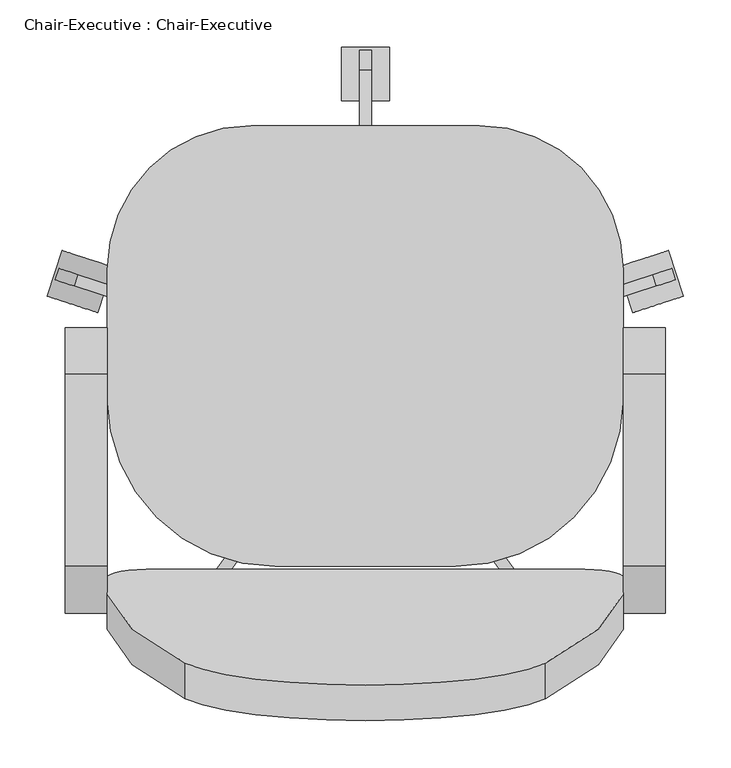
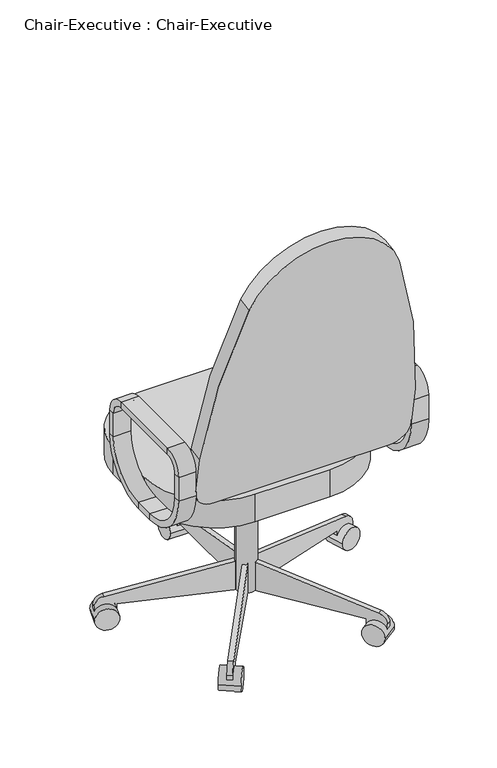
"""IFC4 building model written with IfcOpenShell, lengths in millimetres: furniture geometry, Chair-Executive : Chair-Executive."""

from ifc_helpers import new_model, si_unit, point, frame, frame_2d, origin, place, context, project, spatial, polyline, circle_curve, trimmed, segment, composite_curve, outline, extrude, source, transform, mapped, element, save
from ifc_brep_helpers import plane_surface, cylinder_surface, revolved_surface, advanced_brep


def chair_executive_chair_executive_8d69e98c(model_context):
    return source(origin(), model_context, "Body", "SolidModel", [
        advanced_brep(
        [(-176.5091803, -217.7873012, 546.1), (-176.5091803, -108.0540984, 436.3667972), (-176.5091803, -108.0540984, 420.4917972), (-176.5091803, -233.6623012, 546.1), (-132.0591803, -217.7873012, 546.1), (-132.0591803, -108.0540984, 436.3667972), (-132.0591803, -233.6623012, 546.1), (-132.0591803, -108.0540984, 420.4917972), (-176.5091803, -233.6623012, 609.6), (-176.5091803, -217.7873012, 609.6), (-132.0591803, -217.7873012, 609.6), (-132.0591803, -233.6623012, 609.6), (-176.5091803, -184.2540984, 643.1332028), (-176.5091803, -184.2540984, 659.0082028), (-132.0591803, -184.2540984, 643.1332028), (-132.0591803, -184.2540984, 659.0082028), (-176.5091803, 18.9459016, 659.0082028), (-176.5091803, 18.9459016, 643.1332028), (-132.0591803, 18.9459016, 643.1332028), (-132.0591803, 18.9459016, 659.0082028), (-176.5091803, 52.4791044, 609.6), (-176.5091803, 68.3541044, 609.6), (-132.0591803, 52.4791044, 609.6), (-132.0591803, 68.3541044, 609.6), (-176.5091803, 68.3541044, 546.1), (-176.5091803, 52.4791044, 546.1), (-132.0591803, 52.4791044, 546.1), (-132.0591803, 68.3541044, 546.1), (-176.5091803, -57.2540984, 436.3667972), (-176.5091803, -57.2540984, 420.4917972), (-132.0591803, -57.2540984, 436.3667972), (-132.0591803, -57.2540984, 420.4917972)],
        [
            (0, 1, circle_curve(frame((-176.5091803, -108.0540984, 546.1), z_axis=(1.0, 0.0, 0.0), x_axis=(0.0, 0.0, -1.0)), 109.7332028)),
            (1, 2),
            (2, 3, circle_curve(frame((-176.5091803, -108.0540984, 546.1), z_axis=(-1.0, 0.0, 0.0), x_axis=(0.0, 0.0, -1.0)), 125.6082028)),
            (3, 0),
            (4, 5, circle_curve(frame((-132.0591803, -108.0540984, 546.1), z_axis=(1.0, 0.0, 0.0), x_axis=(0.0, 0.0, -1.0)), 109.7332028)),
            (5, 1),
            (0, 4),
            (6, 7, circle_curve(frame((-132.0591803, -108.0540984, 546.1), z_axis=(1.0, 0.0, 0.0), x_axis=(0.0, 0.0, -1.0)), 125.6082028)),
            (7, 5),
            (4, 6),
            (2, 7),
            (6, 3),
            (3, 8),
            (8, 9),
            (9, 0),
            (9, 10),
            (10, 4),
            (10, 11),
            (11, 6),
            (11, 8),
            (12, 9, circle_curve(frame((-176.5091803, -184.2540984, 609.6), z_axis=(1.0, 0.0, 0.0), x_axis=(0.0, -1.0, 0.0)), 33.5332028)),
            (8, 13, circle_curve(frame((-176.5091803, -184.2540984, 609.6), z_axis=(-1.0, 0.0, 0.0), x_axis=(0.0, -1.0, 0.0)), 49.4082028)),
            (13, 12),
            (14, 10, circle_curve(frame((-132.0591803, -184.2540984, 609.6), z_axis=(1.0, 0.0, 0.0), x_axis=(0.0, -1.0, 0.0)), 33.5332028)),
            (12, 14),
            (15, 11, circle_curve(frame((-132.0591803, -184.2540984, 609.6), z_axis=(1.0, 0.0, 0.0), x_axis=(0.0, -1.0, 0.0)), 49.4082028)),
            (14, 15),
            (15, 13),
            (13, 16),
            (16, 17),
            (17, 12),
            (17, 18),
            (18, 14),
            (18, 19),
            (19, 15),
            (19, 16),
            (20, 17, circle_curve(frame((-176.5091803, 18.9459016, 609.6), z_axis=(1.0, 0.0, 0.0), x_axis=(0.0, 0.0, 1.0)), 33.5332028)),
            (16, 21, circle_curve(frame((-176.5091803, 18.9459016, 609.6), z_axis=(-1.0, 0.0, 0.0), x_axis=(0.0, 0.0, 1.0)), 49.4082028)),
            (21, 20),
            (22, 18, circle_curve(frame((-132.0591803, 18.9459016, 609.6), z_axis=(1.0, 0.0, 0.0), x_axis=(0.0, 0.0, 1.0)), 33.5332028)),
            (20, 22),
            (23, 19, circle_curve(frame((-132.0591803, 18.9459016, 609.6), z_axis=(1.0, 0.0, 0.0), x_axis=(0.0, 0.0, 1.0)), 49.4082028)),
            (22, 23),
            (23, 21),
            (21, 24),
            (24, 25),
            (25, 20),
            (25, 26),
            (26, 22),
            (26, 27),
            (27, 23),
            (27, 24),
            (28, 25, circle_curve(frame((-176.5091803, -57.2540984, 546.1), z_axis=(1.0, 0.0, 0.0), x_axis=(0.0, 1.0, 0.0)), 109.7332028)),
            (24, 29, circle_curve(frame((-176.5091803, -57.2540984, 546.1), z_axis=(-1.0, 0.0, 0.0), x_axis=(0.0, 1.0, 0.0)), 125.6082028)),
            (29, 28),
            (30, 26, circle_curve(frame((-132.0591803, -57.2540984, 546.1), z_axis=(1.0, 0.0, 0.0), x_axis=(0.0, 1.0, 0.0)), 109.7332028)),
            (28, 30),
            (31, 27, circle_curve(frame((-132.0591803, -57.2540984, 546.1), z_axis=(1.0, 0.0, 0.0), x_axis=(0.0, 1.0, 0.0)), 125.6082028)),
            (30, 31),
            (31, 29),
            (29, 2),
            (1, 28),
            (5, 30),
            (7, 31),
        ],
        [
            plane_surface(frame((-176.5091803, -108.0540984, 546.1), z_axis=(-1.0, 0.0, 0.0), x_axis=(0.0, 0.0, -1.0))),
            revolved_surface(polyline([(-176.5091803, -108.0540984, 436.3667972), (-132.0591803, -108.0540984, 436.3667972)]), (-132.0591803, -108.0540984, 546.1), (-1.0, 0.0, 0.0)),
            plane_surface(frame((-132.0591803, -108.0540984, 546.1), z_axis=(1.0, 0.0, 0.0), x_axis=(0.0, 0.0, -1.0))),
            cylinder_surface(frame((-132.0591803, -108.0540984, 546.1), z_axis=(-1.0, 0.0, 0.0), x_axis=(0.0, 0.0, -1.0)), 125.6082028),
            plane_surface(frame((-176.5091803, -233.6623012, 546.1), z_axis=(-1.0, 0.0, 0.0), x_axis=(0.0, 0.0, 1.0))),
            plane_surface(frame((-176.5091803, -217.7873012, 546.1), z_axis=(0.0, 1.0, 0.0), x_axis=(0.0, 0.0, 1.0))),
            plane_surface(frame((-132.0591803, -217.7873012, 546.1), z_axis=(1.0, 0.0, 0.0), x_axis=(0.0, 0.0, 1.0))),
            plane_surface(frame((-132.0591803, -233.6623012, 546.1), z_axis=(0.0, -1.0, 0.0), x_axis=(0.0, 0.0, 1.0))),
            plane_surface(frame((-176.5091803, -184.2540984, 609.6), z_axis=(-1.0, 0.0, 0.0), x_axis=(0.0, -1.0, 0.0))),
            revolved_surface(polyline([(-176.5091803, -217.7873012, 609.6), (-132.0591803, -217.7873012, 609.6)]), (-132.0591803, -184.2540984, 609.6), (-1.0, 0.0, 0.0)),
            plane_surface(frame((-132.0591803, -184.2540984, 609.6), z_axis=(1.0, 0.0, 0.0), x_axis=(0.0, -1.0, 0.0))),
            cylinder_surface(frame((-132.0591803, -184.2540984, 609.6), z_axis=(-1.0, 0.0, 0.0), x_axis=(0.0, -1.0, 0.0)), 49.4082028),
            plane_surface(frame((-176.5091803, -184.2540984, 659.0082028), z_axis=(-1.0, 0.0, 0.0), x_axis=(0.0, 1.0, 0.0))),
            plane_surface(frame((-176.5091803, -184.2540984, 643.1332028), z_axis=(0.0, 0.0, -1.0), x_axis=(0.0, 1.0, 0.0))),
            plane_surface(frame((-132.0591803, -184.2540984, 643.1332028), z_axis=(1.0, 0.0, 0.0), x_axis=(0.0, 1.0, 0.0))),
            plane_surface(frame((-132.0591803, -184.2540984, 659.0082028), z_axis=(0.0, 0.0, 1.0), x_axis=(0.0, 1.0, 0.0))),
            plane_surface(frame((-176.5091803, 18.9459016, 609.6), z_axis=(-1.0, 0.0, 0.0), x_axis=(0.0, 0.0, 1.0))),
            revolved_surface(polyline([(-176.5091803, 18.9459016, 643.1332028), (-132.0591803, 18.9459016, 643.1332028)]), (-132.0591803, 18.9459016, 609.6), (-1.0, 0.0, 0.0)),
            plane_surface(frame((-132.0591803, 18.9459016, 609.6), z_axis=(1.0, 0.0, 0.0), x_axis=(0.0, 0.0, 1.0))),
            cylinder_surface(frame((-132.0591803, 18.9459016, 609.6), z_axis=(-1.0, 0.0, 0.0), x_axis=(0.0, 0.0, 1.0)), 49.4082028),
            plane_surface(frame((-176.5091803, 68.3541044, 609.6), z_axis=(-1.0, 0.0, 0.0), x_axis=(0.0, 0.0, -1.0))),
            plane_surface(frame((-176.5091803, 52.4791044, 609.6), z_axis=(0.0, -1.0, 0.0), x_axis=(0.0, 0.0, -1.0))),
            plane_surface(frame((-132.0591803, 52.4791044, 609.6), z_axis=(1.0, 0.0, 0.0), x_axis=(0.0, 0.0, -1.0))),
            plane_surface(frame((-132.0591803, 68.3541044, 609.6), z_axis=(0.0, 1.0, 0.0), x_axis=(0.0, 0.0, -1.0))),
            plane_surface(frame((-176.5091803, -57.2540984, 546.1), z_axis=(-1.0, 0.0, 0.0), x_axis=(0.0, 1.0, 0.0))),
            revolved_surface(polyline([(-176.5091803, 52.479104400000004, 546.1), (-132.0591803, 52.479104400000004, 546.1)]), (-132.0591803, -57.2540984, 546.1), (-1.0, 0.0, 0.0)),
            plane_surface(frame((-132.0591803, -57.2540984, 546.1), z_axis=(1.0, 0.0, 0.0), x_axis=(0.0, 1.0, 0.0))),
            cylinder_surface(frame((-132.0591803, -57.2540984, 546.1), z_axis=(-1.0, 0.0, 0.0), x_axis=(0.0, 1.0, 0.0)), 125.6082028),
            plane_surface(frame((-176.5091803, -57.2540984, 420.4917972), z_axis=(-1.0, 0.0, 0.0), x_axis=(0.0, -1.0, 0.0))),
            plane_surface(frame((-176.5091803, -57.2540984, 436.3667972), z_axis=(0.0, 0.0, 1.0), x_axis=(0.0, -1.0, 0.0))),
            plane_surface(frame((-132.0591803, -57.2540984, 436.3667972), z_axis=(1.0, 0.0, 0.0), x_axis=(0.0, -1.0, 0.0))),
            plane_surface(frame((-132.0591803, -57.2540984, 420.4917972), z_axis=(0.0, 0.0, -1.0), x_axis=(0.0, -1.0, 0.0))),
        ],
        [
            (0, [[1, 2, 3, 4]]),
            (1, [[5, 6, -1, 7]]),
            (2, [[8, 9, -5, 10]]),
            (3, [[-3, 11, -8, 12]]),
            (4, [[-4, 13, 14, 15]]),
            (5, [[-7, -15, 16, 17]]),
            (6, [[-10, -17, 18, 19]]),
            (7, [[-12, -19, 20, -13]]),
            (8, [[21, -14, 22, 23]]),
            (9, [[24, -16, -21, 25]]),
            (10, [[26, -18, -24, 27]]),
            (11, [[-22, -20, -26, 28]]),
            (12, [[-23, 29, 30, 31]]),
            (13, [[-25, -31, 32, 33]]),
            (14, [[-27, -33, 34, 35]]),
            (15, [[-28, -35, 36, -29]]),
            (16, [[37, -30, 38, 39]]),
            (17, [[40, -32, -37, 41]]),
            (18, [[42, -34, -40, 43]]),
            (19, [[-38, -36, -42, 44]]),
            (20, [[-39, 45, 46, 47]]),
            (21, [[-41, -47, 48, 49]]),
            (22, [[-43, -49, 50, 51]]),
            (23, [[-44, -51, 52, -45]]),
            (24, [[53, -46, 54, 55]]),
            (25, [[56, -48, -53, 57]]),
            (26, [[58, -50, -56, 59]]),
            (27, [[-54, -52, -58, 60]]),
            (28, [[-55, 61, -2, 62]]),
            (29, [[-57, -62, -6, 63]]),
            (30, [[-59, -63, -9, 64]]),
            (31, [[-60, -64, -11, -61]]),
        ],
    ),
        advanced_brep(
        [(414.0408197, -233.6623012, 546.1), (414.0408197, -108.0540984, 420.4917972), (458.4908197, -108.0540984, 420.4917972), (458.4908197, -233.6623012, 546.1), (414.0408197, -217.7873012, 546.1), (414.0408197, -108.0540984, 436.3667972), (458.4908197, -217.7873012, 546.1), (458.4908197, -108.0540984, 436.3667972), (458.4908197, -233.6623012, 609.6), (414.0408197, -233.6623012, 609.6), (414.0408197, -217.7873012, 609.6), (458.4908197, -217.7873012, 609.6), (414.0408197, -184.2540984, 659.0082028), (458.4908197, -184.2540984, 659.0082028), (414.0408197, -184.2540984, 643.1332028), (458.4908197, -184.2540984, 643.1332028), (458.4908197, 18.9459016, 659.0082028), (414.0408197, 18.9459016, 659.0082028), (414.0408197, 18.9459016, 643.1332028), (458.4908197, 18.9459016, 643.1332028), (414.0408197, 68.3541044, 609.6), (458.4908197, 68.3541044, 609.6), (414.0408197, 52.4791044, 609.6), (458.4908197, 52.4791044, 609.6), (458.4908197, 68.3541044, 546.1), (414.0408197, 68.3541044, 546.1), (414.0408197, 52.4791044, 546.1), (458.4908197, 52.4791044, 546.1), (414.0408197, -57.2540984, 420.4917972), (458.4908197, -57.2540984, 420.4917972), (414.0408197, -57.2540984, 436.3667972), (458.4908197, -57.2540984, 436.3667972)],
        [
            (0, 1, circle_curve(frame((414.0408197, -108.0540984, 546.1), z_axis=(1.0, 0.0, 0.0), x_axis=(0.0, 0.0, -1.0)), 125.6082028)),
            (1, 2),
            (2, 3, circle_curve(frame((458.4908197, -108.0540984, 546.1), z_axis=(-1.0, 0.0, 0.0), x_axis=(0.0, 0.0, -1.0)), 125.6082028)),
            (3, 0),
            (4, 5, circle_curve(frame((414.0408197, -108.0540984, 546.1), z_axis=(1.0, 0.0, 0.0), x_axis=(0.0, 0.0, -1.0)), 109.7332028)),
            (5, 1),
            (0, 4),
            (6, 7, circle_curve(frame((458.4908197, -108.0540984, 546.1), z_axis=(1.0, 0.0, 0.0), x_axis=(0.0, 0.0, -1.0)), 109.7332028)),
            (7, 5),
            (4, 6),
            (2, 7),
            (6, 3),
            (3, 8),
            (8, 9),
            (9, 0),
            (9, 10),
            (10, 4),
            (10, 11),
            (11, 6),
            (11, 8),
            (12, 9, circle_curve(frame((414.0408197, -184.2540984, 609.6), z_axis=(1.0, 0.0, 0.0), x_axis=(0.0, -1.0, 0.0)), 49.4082028)),
            (8, 13, circle_curve(frame((458.4908197, -184.2540984, 609.6), z_axis=(-1.0, 0.0, 0.0), x_axis=(0.0, -1.0, 0.0)), 49.4082028)),
            (13, 12),
            (14, 10, circle_curve(frame((414.0408197, -184.2540984, 609.6), z_axis=(1.0, 0.0, 0.0), x_axis=(0.0, -1.0, 0.0)), 33.5332028)),
            (12, 14),
            (15, 11, circle_curve(frame((458.4908197, -184.2540984, 609.6), z_axis=(1.0, 0.0, 0.0), x_axis=(0.0, -1.0, 0.0)), 33.5332028)),
            (14, 15),
            (15, 13),
            (13, 16),
            (16, 17),
            (17, 12),
            (17, 18),
            (18, 14),
            (18, 19),
            (19, 15),
            (19, 16),
            (20, 17, circle_curve(frame((414.0408197, 18.9459016, 609.6), z_axis=(1.0, 0.0, 0.0), x_axis=(0.0, 0.0, 1.0)), 49.4082028)),
            (16, 21, circle_curve(frame((458.4908197, 18.9459016, 609.6), z_axis=(-1.0, 0.0, 0.0), x_axis=(0.0, 0.0, 1.0)), 49.4082028)),
            (21, 20),
            (22, 18, circle_curve(frame((414.0408197, 18.9459016, 609.6), z_axis=(1.0, 0.0, 0.0), x_axis=(0.0, 0.0, 1.0)), 33.5332028)),
            (20, 22),
            (23, 19, circle_curve(frame((458.4908197, 18.9459016, 609.6), z_axis=(1.0, 0.0, 0.0), x_axis=(0.0, 0.0, 1.0)), 33.5332028)),
            (22, 23),
            (23, 21),
            (21, 24),
            (24, 25),
            (25, 20),
            (25, 26),
            (26, 22),
            (26, 27),
            (27, 23),
            (27, 24),
            (28, 25, circle_curve(frame((414.0408197, -57.2540984, 546.1), z_axis=(1.0, 0.0, 0.0), x_axis=(0.0, 1.0, 0.0)), 125.6082028)),
            (24, 29, circle_curve(frame((458.4908197, -57.2540984, 546.1), z_axis=(-1.0, 0.0, 0.0), x_axis=(0.0, 1.0, 0.0)), 125.6082028)),
            (29, 28),
            (30, 26, circle_curve(frame((414.0408197, -57.2540984, 546.1), z_axis=(1.0, 0.0, 0.0), x_axis=(0.0, 1.0, 0.0)), 109.7332028)),
            (28, 30),
            (31, 27, circle_curve(frame((458.4908197, -57.2540984, 546.1), z_axis=(1.0, 0.0, 0.0), x_axis=(0.0, 1.0, 0.0)), 109.7332028)),
            (30, 31),
            (31, 29),
            (29, 2),
            (1, 28),
            (5, 30),
            (7, 31),
        ],
        [
            cylinder_surface(frame((414.0408197, -108.0540984, 546.1), z_axis=(-1.0, 0.0, 0.0), x_axis=(0.0, 0.0, -1.0)), 125.6082028),
            plane_surface(frame((414.0408197, -108.0540984, 546.1), z_axis=(-1.0, 0.0, 0.0), x_axis=(0.0, 0.0, -1.0))),
            revolved_surface(polyline([(414.0408197, -108.0540984, 436.3667972), (458.4908197, -108.0540984, 436.3667972)]), (414.0408197, -108.0540984, 546.1), (-1.0, 0.0, 0.0)),
            plane_surface(frame((458.4908197, -108.0540984, 546.1), z_axis=(1.0, 0.0, 0.0), x_axis=(0.0, 0.0, -1.0))),
            plane_surface(frame((458.4908197, -233.6623012, 546.1), z_axis=(0.0, -1.0, 0.0), x_axis=(0.0, 0.0, 1.0))),
            plane_surface(frame((414.0408197, -233.6623012, 546.1), z_axis=(-1.0, 0.0, 0.0), x_axis=(0.0, 0.0, 1.0))),
            plane_surface(frame((414.0408197, -217.7873012, 546.1), z_axis=(0.0, 1.0, 0.0), x_axis=(0.0, 0.0, 1.0))),
            plane_surface(frame((458.4908197, -217.7873012, 546.1), z_axis=(1.0, 0.0, 0.0), x_axis=(0.0, 0.0, 1.0))),
            cylinder_surface(frame((414.0408197, -184.2540984, 609.6), z_axis=(-1.0, 0.0, 0.0), x_axis=(0.0, -1.0, 0.0)), 49.4082028),
            plane_surface(frame((414.0408197, -184.2540984, 609.6), z_axis=(-1.0, 0.0, 0.0), x_axis=(0.0, -1.0, 0.0))),
            revolved_surface(polyline([(414.0408197, -217.7873012, 609.6), (458.4908197, -217.7873012, 609.6)]), (414.0408197, -184.2540984, 609.6), (-1.0, 0.0, 0.0)),
            plane_surface(frame((458.4908197, -184.2540984, 609.6), z_axis=(1.0, 0.0, 0.0), x_axis=(0.0, -1.0, 0.0))),
            plane_surface(frame((458.4908197, -184.2540984, 659.0082028), z_axis=(0.0, 0.0, 1.0), x_axis=(0.0, 1.0, 0.0))),
            plane_surface(frame((414.0408197, -184.2540984, 659.0082028), z_axis=(-1.0, 0.0, 0.0), x_axis=(0.0, 1.0, 0.0))),
            plane_surface(frame((414.0408197, -184.2540984, 643.1332028), z_axis=(0.0, 0.0, -1.0), x_axis=(0.0, 1.0, 0.0))),
            plane_surface(frame((458.4908197, -184.2540984, 643.1332028), z_axis=(1.0, 0.0, 0.0), x_axis=(0.0, 1.0, 0.0))),
            cylinder_surface(frame((414.0408197, 18.9459016, 609.6), z_axis=(-1.0, 0.0, 0.0), x_axis=(0.0, 0.0, 1.0)), 49.4082028),
            plane_surface(frame((414.0408197, 18.9459016, 609.6), z_axis=(-1.0, 0.0, 0.0), x_axis=(0.0, 0.0, 1.0))),
            revolved_surface(polyline([(414.0408197, 18.9459016, 643.1332028), (458.4908197, 18.9459016, 643.1332028)]), (414.0408197, 18.9459016, 609.6), (-1.0, 0.0, 0.0)),
            plane_surface(frame((458.4908197, 18.9459016, 609.6), z_axis=(1.0, 0.0, 0.0), x_axis=(0.0, 0.0, 1.0))),
            plane_surface(frame((458.4908197, 68.3541044, 609.6), z_axis=(0.0, 1.0, 0.0), x_axis=(0.0, 0.0, -1.0))),
            plane_surface(frame((414.0408197, 68.3541044, 609.6), z_axis=(-1.0, 0.0, 0.0), x_axis=(0.0, 0.0, -1.0))),
            plane_surface(frame((414.0408197, 52.4791044, 609.6), z_axis=(0.0, -1.0, 0.0), x_axis=(0.0, 0.0, -1.0))),
            plane_surface(frame((458.4908197, 52.4791044, 609.6), z_axis=(1.0, 0.0, 0.0), x_axis=(0.0, 0.0, -1.0))),
            cylinder_surface(frame((414.0408197, -57.2540984, 546.1), z_axis=(-1.0, 0.0, 0.0), x_axis=(0.0, 1.0, 0.0)), 125.6082028),
            plane_surface(frame((414.0408197, -57.2540984, 546.1), z_axis=(-1.0, 0.0, 0.0), x_axis=(0.0, 1.0, 0.0))),
            revolved_surface(polyline([(414.0408197, 52.479104400000004, 546.1), (458.4908197, 52.479104400000004, 546.1)]), (414.0408197, -57.2540984, 546.1), (-1.0, 0.0, 0.0)),
            plane_surface(frame((458.4908197, -57.2540984, 546.1), z_axis=(1.0, 0.0, 0.0), x_axis=(0.0, 1.0, 0.0))),
            plane_surface(frame((458.4908197, -57.2540984, 420.4917972), z_axis=(0.0, 0.0, -1.0), x_axis=(0.0, -1.0, 0.0))),
            plane_surface(frame((414.0408197, -57.2540984, 420.4917972), z_axis=(-1.0, 0.0, 0.0), x_axis=(0.0, -1.0, 0.0))),
            plane_surface(frame((414.0408197, -57.2540984, 436.3667972), z_axis=(0.0, 0.0, 1.0), x_axis=(0.0, -1.0, 0.0))),
            plane_surface(frame((458.4908197, -57.2540984, 436.3667972), z_axis=(1.0, 0.0, 0.0), x_axis=(0.0, -1.0, 0.0))),
        ],
        [
            (0, [[1, 2, 3, 4]]),
            (1, [[5, 6, -1, 7]]),
            (2, [[8, 9, -5, 10]]),
            (3, [[-3, 11, -8, 12]]),
            (4, [[-4, 13, 14, 15]]),
            (5, [[-7, -15, 16, 17]]),
            (6, [[-10, -17, 18, 19]]),
            (7, [[-12, -19, 20, -13]]),
            (8, [[21, -14, 22, 23]]),
            (9, [[24, -16, -21, 25]]),
            (10, [[26, -18, -24, 27]]),
            (11, [[-22, -20, -26, 28]]),
            (12, [[-23, 29, 30, 31]]),
            (13, [[-25, -31, 32, 33]]),
            (14, [[-27, -33, 34, 35]]),
            (15, [[-28, -35, 36, -29]]),
            (16, [[37, -30, 38, 39]]),
            (17, [[40, -32, -37, 41]]),
            (18, [[42, -34, -40, 43]]),
            (19, [[-38, -36, -42, 44]]),
            (20, [[-39, 45, 46, 47]]),
            (21, [[-41, -47, 48, 49]]),
            (22, [[-43, -49, 50, 51]]),
            (23, [[-44, -51, 52, -45]]),
            (24, [[53, -46, 54, 55]]),
            (25, [[56, -48, -53, 57]]),
            (26, [[58, -50, -56, 59]]),
            (27, [[-54, -52, -58, 60]]),
            (28, [[-55, 61, -2, 62]]),
            (29, [[-57, -62, -6, 63]]),
            (30, [[-59, -63, -9, 64]]),
            (31, [[-60, -64, -11, -61]]),
        ],
    ),
        extrude(outline(composite_curve([segment(trimmed(circle_curve(frame_2d((0.0, -50.8)), 50.8), [point((0.0, 0.0))], [point((50.8, -50.8))], False, "CARTESIAN"), True, "CONTINUOUS"), segment(polyline([(50.8, -50.8), (50.8, -152.4)]), True, "CONTINUOUS"), segment(trimmed(circle_curve(frame_2d((-1471.2021854, -74.3913617)), 1524.0), [point((50.8, -152.4))], [point((-31.75, -574.9444618))], False, "CARTESIAN"), True, "CONTINUOUS"), segment(trimmed(circle_curve(frame_2d((-222.25, -504.2338544)), 203.2), [point((-31.75, -574.9444618))], [point((-412.75, -574.9444618))], False, "CARTESIAN"), True, "CONTINUOUS"), segment(trimmed(circle_curve(frame_2d((1026.7021854, -74.3913617)), 1524.0), [point((-412.75, -574.9444618))], [point((-495.3, -152.4))], False, "CARTESIAN"), True, "CONTINUOUS"), segment(polyline([(-495.3, -152.4), (-495.3, -50.8)]), True, "CONTINUOUS"), segment(trimmed(circle_curve(frame_2d((-444.5, -50.8)), 50.8), [point((-495.3, -50.8))], [point((-444.5, 0.0))], False, "CARTESIAN"), True, "CONTINUOUS"), segment(polyline([(-444.5, 0.0), (0.0, 0.0)]), True, "CONTINUOUS")], self_intersect=False)), frame((363.2408197, -224.5698964, 503.1641822), z_axis=(0.0, 0.9848077530122084, 0.17364817766692853), x_axis=(1.0, 0.0, 0.0)), (0.0, 0.0, 1.0), 38.1),
        extrude(outline(composite_curve([segment(trimmed(circle_curve(frame_2d((20.3408197, 129.4961016)), 152.4), [point((-132.0591803, 129.4961016))], [point((20.3408197, 281.8961016))], False, "CARTESIAN"), True, "CONTINUOUS"), segment(polyline([(20.3408197, 281.8961016), (261.6408197, 281.8961016)]), True, "CONTINUOUS"), segment(trimmed(circle_curve(frame_2d((261.6408197, 129.4961016)), 152.4), [point((261.6408197, 281.8961016))], [point((414.0408197, 129.4961016))], False, "CARTESIAN"), True, "CONTINUOUS"), segment(polyline([(414.0408197, 129.4961016), (414.0408197, -6.4540984)]), True, "CONTINUOUS"), segment(trimmed(circle_curve(frame_2d((236.2408197, -6.4540984)), 177.8), [point((414.0408197, -6.4540984))], [point((236.2408197, -184.2540984))], False, "CARTESIAN"), True, "CONTINUOUS"), segment(polyline([(236.2408197, -184.2540984), (45.7408197, -184.2540984)]), True, "CONTINUOUS"), segment(trimmed(circle_curve(frame_2d((45.7408197, -6.4540984)), 177.8), [point((45.7408197, -184.2540984))], [point((-132.0591803, -6.4540984))], False, "CARTESIAN"), True, "CONTINUOUS"), segment(polyline([(-132.0591803, -6.4540984), (-132.0591803, 129.4961016)]), True, "CONTINUOUS")], self_intersect=False)), frame((0.0, 0.0, 383.7835944), z_axis=(0.0, 0.0, 1.0), x_axis=(1.0, 0.0, 0.0)), (0.0, 0.0, 1.0), 73.4164056),
        extrude(outline(composite_curve([segment(trimmed(circle_curve(frame_2d((140.9908197, 18.9459016)), 25.4), [point((115.5908197, 18.9459016))], [point((166.3908197, 18.9459016))], False, "CARTESIAN"), True, "CONTINUOUS"), segment(trimmed(circle_curve(frame_2d((140.9908197, 18.9459016)), 25.4), [point((166.3908197, 18.9459016))], [point((115.5908197, 18.9459016))], False, "CARTESIAN"), True, "CONTINUOUS")], self_intersect=False)), frame((0.0, 0.0, 53.5835944), z_axis=(0.0, 0.0, 1.0), x_axis=(1.0, 0.0, 0.0)), (0.0, 0.0, 1.0), 330.5914056),
        extrude(outline(composite_curve([segment(trimmed(circle_curve(frame_2d((0.0, -28.2002727)), 28.2002727), [point((0.0, -56.4005455))], [point((0.0, 0.0))], False, "CARTESIAN"), True, "CONTINUOUS"), segment(trimmed(circle_curve(frame_2d((0.0, -28.2002727)), 28.2002727), [point((0.0, 0.0))], [point((0.0, -56.4005455))], False, "CARTESIAN"), True, "CONTINUOUS")], self_intersect=False)), frame((477.6203484, 101.6163254, 28.1835944), z_axis=(-0.3090169943749423, 0.9510565162951553, 0.0), x_axis=(0.0, 0.0, 1.0)), (0.0, 0.0, 1.0), 50.8),
        extrude(outline(composite_curve([segment(polyline([(-25.4, 0.0), (0.0, 0.0), (0.0, -50.8), (-24.303053, -50.8)]), True, "CONTINUOUS"), segment(trimmed(circle_curve(frame_2d((-24.303053, -25.4)), 25.4), [point((-24.303053, -50.8))], [point((-49.3171699, -29.8106637))], False, "CARTESIAN"), True, "CONTINUOUS"), segment(polyline([(-49.3171699, -29.8106637), (-101.6, 266.7), (-101.6, 292.1), (-25.4, 292.1), (-25.4, 0.0)]), True, "CONTINUOUS")], self_intersect=False)), frame((420.756686, 103.1705568, 28.1835944), z_axis=(-0.3090169943749423, 0.9510565162951553, 0.0), x_axis=(0.0, 0.0, -1.0)), (0.0, 0.0, 1.0), 12.7),
        extrude(outline(composite_curve([segment(trimmed(circle_curve(frame_2d((0.0, -28.2002727)), 28.2002727), [point((0.0, -56.4005455))], [point((0.0, 0.0))], False, "CARTESIAN"), True, "CONTINUOUS"), segment(trimmed(circle_curve(frame_2d((0.0, -28.2002727)), 28.2002727), [point((0.0, 0.0))], [point((0.0, -56.4005455))], False, "CARTESIAN"), True, "CONTINUOUS")], self_intersect=False)), frame((323.63931, -275.6612394, 28.1835944), z_axis=(0.8090169943749499, 0.5877852522924699, 0.0), x_axis=(0.0, 0.0, 1.0)), (0.0, 0.0, 1.0), 50.8),
        extrude(outline(composite_curve([segment(polyline([(-25.4, 0.0), (0.0, 0.0), (0.0, -50.8), (-24.303053, -50.8)]), True, "CONTINUOUS"), segment(trimmed(circle_curve(frame_2d((-24.303053, -25.3999999)), 25.4), [point((-24.303053, -50.8))], [point((-49.3171699, -29.8106636))], False, "CARTESIAN"), True, "CONTINUOUS"), segment(polyline([(-49.3171699, -29.8106636), (-101.6, 266.7), (-101.6, 292.1), (-25.4, 292.1), (-25.4, 0.0)]), True, "CONTINUOUS")], self_intersect=False)), frame((307.545634, -221.1003988, 28.1835944), z_axis=(0.8090169943749499, 0.5877852522924699, 0.0), x_axis=(0.0, 0.0, -1.0)), (0.0, 0.0, 1.0), 12.7),
        extrude(outline(composite_curve([segment(trimmed(circle_curve(frame_2d((0.0, -28.2002727)), 28.2002727), [point((0.0, -56.4005455))], [point((0.0, 0.0))], False, "CARTESIAN"), True, "CONTINUOUS"), segment(trimmed(circle_curve(frame_2d((0.0, -28.2002727)), 28.2002727), [point((0.0, 0.0))], [point((0.0, -56.4005455))], False, "CARTESIAN"), True, "CONTINUOUS")], self_intersect=False)), frame((-41.6576707, -275.6612394, 28.1835944), z_axis=(-0.8090169943749458, 0.5877852522924754, 0.0), x_axis=(0.0, 0.0, -1.0)), (0.0, 0.0, 1.0), 50.8),
        extrude(outline(composite_curve([segment(polyline([(25.4, 0.0), (25.4, 292.1), (101.6, 292.1), (101.6, 266.7), (49.3171699, -29.8106637)]), True, "CONTINUOUS"), segment(trimmed(circle_curve(frame_2d((24.303053, -25.3999999)), 25.4), [point((49.3171699, -29.8106637))], [point((24.303053, -50.8))], False, "CARTESIAN"), True, "CONTINUOUS"), segment(polyline([(24.303053, -50.8), (0.0, -50.8), (0.0, 0.0), (25.4, 0.0)]), True, "CONTINUOUS")], self_intersect=False)), frame((-25.5639946, -221.1003988, 28.1835944), z_axis=(-0.8090169943749459, 0.5877852522924754, 0.0), x_axis=(0.0, 0.0, 1.0)), (0.0, 0.0, 1.0), 12.7),
        extrude(outline(composite_curve([segment(trimmed(circle_curve(frame_2d((0.0, -28.2002727)), 28.2002727), [point((0.0, -56.4005454))], [point((0.0, 0.0))], False, "CARTESIAN"), True, "CONTINUOUS"), segment(trimmed(circle_curve(frame_2d((0.0, -28.2002727)), 28.2002727), [point((0.0, 0.0))], [point((0.0, -56.4005454))], False, "CARTESIAN"), True, "CONTINUOUS")], self_intersect=False)), frame((-195.638709, 101.6163254, 28.1835944), z_axis=(0.3090169943749487, 0.9510565162951532, 0.0), x_axis=(0.0, 0.0, -1.0)), (0.0, 0.0, 1.0), 50.8),
        extrude(outline(composite_curve([segment(polyline([(25.4, 0.0), (25.4, 292.1000001), (101.6, 292.1000001), (101.6, 266.7), (49.3171699, -29.8106636)]), True, "CONTINUOUS"), segment(trimmed(circle_curve(frame_2d((24.303053, -25.4)), 25.4), [point((49.3171699, -29.8106636))], [point((24.303053, -50.8))], False, "CARTESIAN"), True, "CONTINUOUS"), segment(polyline([(24.303053, -50.8), (0.0, -50.8), (0.0, 0.0), (25.4, 0.0)]), True, "CONTINUOUS")], self_intersect=False)), frame((-138.7750467, 103.1705568, 28.1835944), z_axis=(0.3090169943749487, 0.9510565162951532, 0.0), x_axis=(0.0, 0.0, 1.0)), (0.0, 0.0, 1.0), 12.7),
        extrude(outline(composite_curve([segment(trimmed(circle_curve(frame_2d((336.4459016, 28.1835944)), 28.2002727), [point((308.2456289, 28.1835944))], [point((364.6461744, 28.1835944))], False, "CARTESIAN"), True, "CONTINUOUS"), segment(trimmed(circle_curve(frame_2d((336.4459016, 28.1835944)), 28.2002727), [point((364.6461744, 28.1835944))], [point((308.2456289, 28.1835944))], False, "CARTESIAN"), True, "CONTINUOUS")], self_intersect=False)), frame((115.5908197, 0.0, 0.0), z_axis=(1.0, 0.0, 0.0), x_axis=(0.0, 1.0, 0.0)), (0.0, 0.0, 1.0), 50.8),
        extrude(outline(composite_curve([segment(polyline([(311.0459016, 53.5835944), (18.9459016, 53.5835944), (18.9459016, 129.7835944), (44.3459016, 129.7835944), (340.8565654, 77.5007643)]), True, "CONTINUOUS"), segment(trimmed(circle_curve(frame_2d((336.4459016, 52.4866474)), 25.4), [point((340.8565654, 77.5007643))], [point((361.8459016, 52.4866474))], False, "CARTESIAN"), True, "CONTINUOUS"), segment(polyline([(361.8459016, 52.4866474), (361.8459016, 28.1835944), (311.0459016, 28.1835944), (311.0459016, 53.5835944)]), True, "CONTINUOUS")], self_intersect=False)), frame((134.6408197, 0.0, 0.0), z_axis=(1.0, 0.0, 0.0), x_axis=(0.0, 1.0, 0.0)), (0.0, 0.0, 1.0), 12.7),
        extrude(outline(polyline([(69.7459016, 383.7835944), (69.7459016, 371.0835944), (18.9459016, 283.0954134), (-19.1540984, 283.0954134), (-19.1540984, 383.7835944), (69.7459016, 383.7835944)])), frame((90.1908197, 0.0, 0.0), z_axis=(1.0, 0.0, 0.0), x_axis=(0.0, 1.0, 0.0)), (0.0, 0.0, 1.0), 101.6),
    ])


if __name__ == "__main__":
    model = new_model("IFC4")
    model_context = context("Model", 3, world=origin())
    ifc_project = project(units=[si_unit("LENGTHUNIT", "METRE", prefix="MILLI")], contexts=[model_context])
    site = spatial("IfcSite", under=ifc_project)
    building = spatial("IfcBuilding", under=site)
    placement = place(None, origin())
    chair_executive_chair_executive_shape = chair_executive_chair_executive_8d69e98c(model_context)
    element("IfcFurniture", 1, ObjectType="Chair-Executive : Chair-Executive", at=placement, inside=building, context=model_context, shape_type="MappedRepresentation", body=[
        mapped(chair_executive_chair_executive_shape, transform((0.0, 0.0, 0.0), x_axis=(1.0, 0.0, 0.0), y_axis=(0.0, 1.0, 0.0), z_axis=(0.0, 0.0, 1.0))),
    ])
    save(model, "model.ifc")

# Revit data of these elements
# Type "Chair-Executive : Chair-Executive"
#   Assembly Code = "E2020200"
#   Base/Arms Material = Plastic, Opaque Black
#   Casters Material = Plastic, Opaque Black
#   Seat/Back Material = Textile - Slate Blue
#   Default Elevation = 0
# Element 1 (IfcFurniture, "Chair-Executive : Chair-Executive")
#   Materials on its faces: "Plastic, Opaque Black", "Textile - Slate Blue"
# Materials
#   "Plastic, Opaque Black": class "Plastic", colour RGB 0 0 0, transparency 0.7, Description = "Plastic, generic, opaque black", Cost = 0
#   "Textile - Slate Blue": class "Fabric", colour RGB 98 102 118, transparency 0
